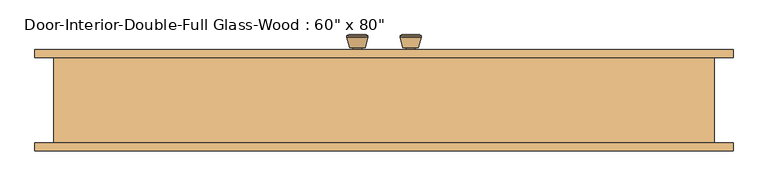
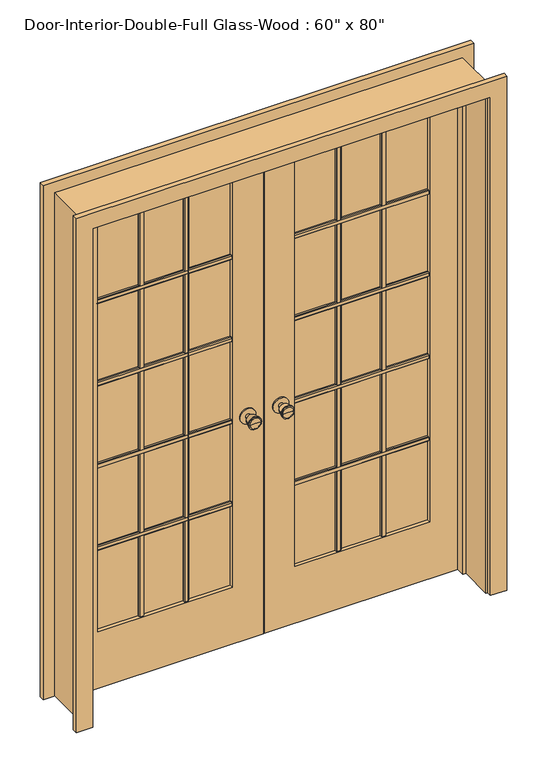
"""IFC4 building model written with IfcOpenShell, lengths in millimetres: door geometry."""

from ifc_helpers import new_model, si_unit, point, frame, frame_2d, origin, place, context, project, spatial, polyline, circle_curve, trimmed, segment, composite_curve, outline, extrude, faceted_brep, source, transform, mapped, element, save
from ifc_brep_helpers import plane_surface, cylinder_surface, revolved_surface, advanced_brep


def door_9d00318c(model_context):
    return source(origin(), model_context, "Body", "SolidModel", [
        advanced_brep(
        [(-63.5, 104.425, 914.4), (-73.5, 104.425, 914.4), (-53.5, 104.425, 914.4), (-83.9758676, 153.425, 914.4), (-63.5, 153.425, 914.4), (-43.0241324, 153.425, 914.4), (-88.5, 151.5971319, 914.4), (-38.5, 151.5971319, 914.4), (-88.5, 148.1334537, 914.4), (-38.5, 148.1334537, 914.4), (-82.136236, 123.425, 914.4), (-44.863764, 123.425, 914.4), (-73.5, 123.425, 914.4), (-53.5, 123.425, 914.4)],
        [
            (0, 1),
            (1, 2, circle_curve(frame((-63.5, 104.425, 914.4), z_axis=(0.0, -1.0, 0.0), x_axis=(1.0, 0.0, 0.0)), 10.0)),
            (2, 0),
            (2, 1, circle_curve(frame((-63.5, 104.425, 914.4), z_axis=(0.0, -1.0, 0.0), x_axis=(1.0, 0.0, 0.0)), 10.0)),
            (3, 4),
            (4, 5),
            (5, 3, circle_curve(frame((-63.5, 153.425, 914.4), z_axis=(0.0, 1.0, 0.0), x_axis=(1.0, 0.0, 0.0)), 20.4758676)),
            (3, 5, circle_curve(frame((-63.5, 153.425, 914.4), z_axis=(0.0, 1.0, 0.0), x_axis=(1.0, 0.0, 0.0)), 20.4758676)),
            (6, 3),
            (5, 7),
            (7, 6, circle_curve(frame((-63.5, 151.5971319, 914.4), z_axis=(0.0, 1.0, 0.0), x_axis=(1.0, 0.0, 0.0)), 25.0)),
            (6, 7, circle_curve(frame((-63.5, 151.5971319, 914.4), z_axis=(0.0, 1.0, 0.0), x_axis=(1.0, 0.0, 0.0)), 25.0)),
            (8, 6),
            (7, 9),
            (9, 8, circle_curve(frame((-63.5, 148.1334537, 914.4), z_axis=(0.0, 1.0, 0.0), x_axis=(1.0, 0.0, 0.0)), 25.0)),
            (8, 9, circle_curve(frame((-63.5, 148.1334537, 914.4), z_axis=(0.0, 1.0, 0.0), x_axis=(1.0, 0.0, 0.0)), 25.0)),
            (10, 8),
            (9, 11),
            (11, 10, circle_curve(frame((-63.5, 123.425, 914.4), z_axis=(0.0, 1.0, 0.0), x_axis=(1.0, 0.0, 0.0)), 18.636236)),
            (10, 11, circle_curve(frame((-63.5, 123.425, 914.4), z_axis=(0.0, 1.0, 0.0), x_axis=(1.0, 0.0, 0.0)), 18.636236)),
            (12, 10),
            (11, 13),
            (13, 12, circle_curve(frame((-63.5, 123.425, 914.4), z_axis=(0.0, 1.0, 0.0), x_axis=(1.0, 0.0, 0.0)), 10.0)),
            (12, 13, circle_curve(frame((-63.5, 123.425, 914.4), z_axis=(0.0, 1.0, 0.0), x_axis=(1.0, 0.0, 0.0)), 10.0)),
            (1, 12),
            (13, 2),
        ],
        [
            plane_surface(frame((-63.5, 104.425, 914.4), z_axis=(0.0, -1.0, 0.0), x_axis=(1.0, 0.0, 0.0))),
            plane_surface(frame((-63.5, 153.425, 914.4), z_axis=(0.0, 1.0, 0.0), x_axis=(1.0, 0.0, 0.0))),
            revolved_surface(polyline([(-43.0241324, 153.425, 914.4), (-38.5, 151.5971319, 914.4)]), (-63.5, 104.425, 914.4), (0.0, -1.0, 0.0)),
            cylinder_surface(frame((-63.5, 104.425, 914.4), z_axis=(0.0, -1.0, 0.0), x_axis=(1.0, 0.0, 0.0)), 25.0),
            revolved_surface(polyline([(-38.5, 148.1334537, 914.4), (-44.863764, 123.425, 914.4)]), (-63.5, 104.425, 914.4), (0.0, -1.0, 0.0)),
            plane_surface(frame((-63.5, 123.425, 914.4), z_axis=(0.0, -1.0, 0.0), x_axis=(1.0, 0.0, 0.0))),
            cylinder_surface(frame((-63.5, 104.425, 914.4), z_axis=(0.0, -1.0, 0.0), x_axis=(1.0, 0.0, 0.0)), 10.0),
        ],
        [
            (0, [[1, 2, 3]]),
            (0, [[-3, 4, -1]]),
            (1, [[5, 6, 7]]),
            (1, [[-6, -5, 8]]),
            (2, [[9, -7, 10, 11]]),
            (2, [[-10, -8, -9, 12]]),
            (3, [[13, -11, 14, 15]]),
            (3, [[-14, -12, -13, 16]]),
            (4, [[17, -15, 18, 19]]),
            (4, [[-18, -16, -17, 20]]),
            (5, [[21, -19, 22, 23]]),
            (5, [[-22, -20, -21, 24]]),
            (6, [[25, -23, 26, -2]]),
            (6, [[-26, -24, -25, -4]]),
        ],
    ),
        extrude(outline(composite_curve([segment(trimmed(circle_curve(frame_2d((914.4, -63.5)), 30.0), [point((914.4, -33.5))], [point((914.4, -93.5))], False, "CARTESIAN"), True, "CONTINUOUS"), segment(trimmed(circle_curve(frame_2d((914.4, -63.5)), 30.0), [point((914.4, -93.5))], [point((914.4, -33.5))], False, "CARTESIAN"), True, "CONTINUOUS")], self_intersect=False)), frame((0.0, 98.425, 0.0), z_axis=(0.0, 1.0, 0.0), x_axis=(0.0, 0.0, 1.0)), (0.0, 0.0, 1.0), 6.0),
        advanced_brep(
        [(-63.5, 57.5, 914.4), (-53.5, 57.5, 914.4), (-73.5, 57.5, 914.4), (-83.9758676, 8.5, 914.4), (-43.0241324, 8.5, 914.4), (-63.5, 8.5, 914.4), (-88.5, 10.3278681, 914.4), (-38.5, 10.3278681, 914.4), (-88.5, 13.7915463, 914.4), (-38.5, 13.7915463, 914.4), (-82.136236, 38.5, 914.4), (-44.863764, 38.5, 914.4), (-73.5, 38.5, 914.4), (-53.5, 38.5, 914.4)],
        [
            (0, 1),
            (1, 2, circle_curve(frame((-63.5, 57.5, 914.4), z_axis=(0.0, 1.0, 0.0), x_axis=(1.0, 0.0, 0.0)), 10.0)),
            (2, 0),
            (2, 1, circle_curve(frame((-63.5, 57.5, 914.4), z_axis=(0.0, 1.0, 0.0), x_axis=(1.0, 0.0, 0.0)), 10.0)),
            (3, 4, circle_curve(frame((-63.5, 8.5, 914.4), z_axis=(0.0, -1.0, 0.0), x_axis=(1.0, 0.0, 0.0)), 20.4758676)),
            (4, 5),
            (5, 3),
            (4, 3, circle_curve(frame((-63.5, 8.5, 914.4), z_axis=(0.0, -1.0, 0.0), x_axis=(1.0, 0.0, 0.0)), 20.4758676)),
            (6, 7, circle_curve(frame((-63.5, 10.3278681, 914.4), z_axis=(0.0, -1.0, 0.0), x_axis=(1.0, 0.0, 0.0)), 25.0)),
            (7, 4),
            (3, 6),
            (7, 6, circle_curve(frame((-63.5, 10.3278681, 914.4), z_axis=(0.0, -1.0, 0.0), x_axis=(1.0, 0.0, 0.0)), 25.0)),
            (8, 9, circle_curve(frame((-63.5, 13.7915463, 914.4), z_axis=(0.0, -1.0, 0.0), x_axis=(1.0, 0.0, 0.0)), 25.0)),
            (9, 7),
            (6, 8),
            (9, 8, circle_curve(frame((-63.5, 13.7915463, 914.4), z_axis=(0.0, -1.0, 0.0), x_axis=(1.0, 0.0, 0.0)), 25.0)),
            (10, 11, circle_curve(frame((-63.5, 38.5, 914.4), z_axis=(0.0, -1.0, 0.0), x_axis=(1.0, 0.0, 0.0)), 18.636236)),
            (11, 9),
            (8, 10),
            (11, 10, circle_curve(frame((-63.5, 38.5, 914.4), z_axis=(0.0, -1.0, 0.0), x_axis=(1.0, 0.0, 0.0)), 18.636236)),
            (12, 13, circle_curve(frame((-63.5, 38.5, 914.4), z_axis=(0.0, -1.0, 0.0), x_axis=(1.0, 0.0, 0.0)), 10.0)),
            (13, 11),
            (10, 12),
            (13, 12, circle_curve(frame((-63.5, 38.5, 914.4), z_axis=(0.0, -1.0, 0.0), x_axis=(1.0, 0.0, 0.0)), 10.0)),
            (1, 13),
            (12, 2),
        ],
        [
            plane_surface(frame((-63.5, 57.5, 914.4), z_axis=(0.0, 1.0, 0.0), x_axis=(1.0, 0.0, 0.0))),
            plane_surface(frame((-63.5, 8.5, 914.4), z_axis=(0.0, -1.0, 0.0), x_axis=(1.0, 0.0, 0.0))),
            revolved_surface(polyline([(-43.0241324, 8.5, 914.4), (-38.5, 10.3278681, 914.4)]), (-63.5, 57.5, 914.4), (0.0, 1.0, 0.0)),
            cylinder_surface(frame((-63.5, 57.5, 914.4), z_axis=(0.0, 1.0, 0.0), x_axis=(1.0, 0.0, 0.0)), 25.0),
            revolved_surface(polyline([(-38.5, 13.7915463, 914.4), (-44.863764, 38.5, 914.4)]), (-63.5, 57.5, 914.4), (0.0, 1.0, 0.0)),
            plane_surface(frame((-63.5, 38.5, 914.4), z_axis=(0.0, 1.0, 0.0), x_axis=(1.0, 0.0, 0.0))),
            cylinder_surface(frame((-63.5, 57.5, 914.4), z_axis=(0.0, 1.0, 0.0), x_axis=(1.0, 0.0, 0.0)), 10.0),
        ],
        [
            (0, [[1, 2, 3]]),
            (0, [[-3, 4, -1]]),
            (1, [[5, 6, 7]]),
            (1, [[8, -7, -6]]),
            (2, [[9, 10, -5, 11]]),
            (2, [[12, -11, -8, -10]]),
            (3, [[13, 14, -9, 15]]),
            (3, [[16, -15, -12, -14]]),
            (4, [[17, 18, -13, 19]]),
            (4, [[20, -19, -16, -18]]),
            (5, [[21, 22, -17, 23]]),
            (5, [[24, -23, -20, -22]]),
            (6, [[-2, 25, -21, 26]]),
            (6, [[-4, -26, -24, -25]]),
        ],
    ),
        extrude(outline(composite_curve([segment(trimmed(circle_curve(frame_2d((914.4, -63.5)), 30.0), [point((914.4, -33.5))], [point((914.4, -93.5))], False, "CARTESIAN"), True, "CONTINUOUS"), segment(trimmed(circle_curve(frame_2d((914.4, -63.5)), 30.0), [point((914.4, -93.5))], [point((914.4, -33.5))], False, "CARTESIAN"), True, "CONTINUOUS")], self_intersect=False)), frame((0.0, 57.5, 0.0), z_axis=(0.0, 1.0, 0.0), x_axis=(0.0, 0.0, 1.0)), (0.0, 0.0, 1.0), 6.0),
        extrude(outline(polyline([(77.47, 1586.23), (77.47, 1567.18), (71.12, 1567.18), (67.945, 1570.355), (67.945, 1583.055), (71.12, 1586.23), (77.47, 1586.23)])), frame((120.65, 0.0, 0.0), z_axis=(1.0, 0.0, 0.0), x_axis=(0.0, 1.0, 0.0)), (0.0, 0.0, 1.0), 520.7),
        extrude(outline(polyline([(77.47, 1249.9975), (77.47, 1230.9475), (71.12, 1230.9475), (67.945, 1234.1225), (67.945, 1246.8225), (71.12, 1249.9975), (77.47, 1249.9975)])), frame((120.65, 0.0, 0.0), z_axis=(1.0, 0.0, 0.0), x_axis=(0.0, 1.0, 0.0)), (0.0, 0.0, 1.0), 520.7),
        extrude(outline(polyline([(77.47, 913.765), (77.47, 894.715), (71.12, 894.715), (67.945, 897.89), (67.945, 910.59), (71.12, 913.765), (77.47, 913.765)])), frame((120.65, 0.0, 0.0), z_axis=(1.0, 0.0, 0.0), x_axis=(0.0, 1.0, 0.0)), (0.0, 0.0, 1.0), 520.7),
        extrude(outline(polyline([(77.47, 577.5325), (77.47, 558.4825), (71.12, 558.4825), (67.945, 561.6575), (67.945, 574.3575), (71.12, 577.5325), (77.47, 577.5325)])), frame((120.65, 0.0, 0.0), z_axis=(1.0, 0.0, 0.0), x_axis=(0.0, 1.0, 0.0)), (0.0, 0.0, 1.0), 520.7),
        extrude(outline(polyline([(458.2583333, 77.47), (477.3083333, 77.47), (477.3083333, 71.12), (474.1333333, 67.945), (461.4333333, 67.945), (458.2583333, 71.12), (458.2583333, 77.47)])), frame((0.0, 0.0, 231.775), z_axis=(0.0, 0.0, 1.0), x_axis=(1.0, 0.0, 0.0)), (0.0, 0.0, 1.0), 1681.1625),
        extrude(outline(polyline([(284.6916667, 77.47), (303.7416667, 77.47), (303.7416667, 71.12), (300.5666667, 67.945), (287.8666667, 67.945), (284.6916667, 71.12), (284.6916667, 77.47)])), frame((0.0, 0.0, 231.775), z_axis=(0.0, 0.0, 1.0), x_axis=(1.0, 0.0, 0.0)), (0.0, 0.0, 1.0), 1681.1625),
        extrude(outline(polyline([(84.455, 1586.23), (90.805, 1586.23), (93.98, 1583.055), (93.98, 1570.355), (90.805, 1567.18), (84.455, 1567.18), (84.455, 1586.23)])), frame((-641.35, 0.0, 0.0), z_axis=(1.0, 0.0, 0.0), x_axis=(0.0, 1.0, 0.0)), (0.0, 0.0, 1.0), 520.7),
        extrude(outline(polyline([(84.455, 1249.9975), (90.805, 1249.9975), (93.98, 1246.8225), (93.98, 1234.1225), (90.805, 1230.9475), (84.455, 1230.9475), (84.455, 1249.9975)])), frame((-641.35, 0.0, 0.0), z_axis=(1.0, 0.0, 0.0), x_axis=(0.0, 1.0, 0.0)), (0.0, 0.0, 1.0), 520.7),
        extrude(outline(polyline([(84.455, 913.765), (90.805, 913.765), (93.98, 910.59), (93.98, 897.89), (90.805, 894.715), (84.455, 894.715), (84.455, 913.765)])), frame((-641.35, 0.0, 0.0), z_axis=(1.0, 0.0, 0.0), x_axis=(0.0, 1.0, 0.0)), (0.0, 0.0, 1.0), 520.7),
        extrude(outline(polyline([(84.455, 577.5325), (90.805, 577.5325), (93.98, 574.3575), (93.98, 561.6575), (90.805, 558.4825), (84.455, 558.4825), (84.455, 577.5325)])), frame((-641.35, 0.0, 0.0), z_axis=(1.0, 0.0, 0.0), x_axis=(0.0, 1.0, 0.0)), (0.0, 0.0, 1.0), 520.7),
        extrude(outline(polyline([(-303.7416667, 84.455), (-303.7416667, 90.805), (-300.5666667, 93.98), (-287.8666667, 93.98), (-284.6916667, 90.805), (-284.6916667, 84.455), (-303.7416667, 84.455)])), frame((0.0, 0.0, 231.775), z_axis=(0.0, 0.0, 1.0), x_axis=(1.0, 0.0, 0.0)), (0.0, 0.0, 1.0), 1681.1625),
        extrude(outline(polyline([(-477.3083333, 84.455), (-477.3083333, 90.805), (-474.1333333, 93.98), (-461.4333333, 93.98), (-458.2583333, 90.805), (-458.2583333, 84.455), (-477.3083333, 84.455)])), frame((0.0, 0.0, 231.775), z_axis=(0.0, 0.0, 1.0), x_axis=(1.0, 0.0, 0.0)), (0.0, 0.0, 1.0), 1681.1625),
        extrude(outline(polyline([(84.455, 1586.23), (90.805, 1586.23), (93.98, 1583.055), (93.98, 1570.355), (90.805, 1567.18), (84.455, 1567.18), (84.455, 1586.23)])), frame((120.65, 0.0, 0.0), z_axis=(1.0, 0.0, 0.0), x_axis=(0.0, 1.0, 0.0)), (0.0, 0.0, 1.0), 520.7),
        extrude(outline(polyline([(84.455, 1249.9975), (90.805, 1249.9975), (93.98, 1246.8225), (93.98, 1234.1225), (90.805, 1230.9475), (84.455, 1230.9475), (84.455, 1249.9975)])), frame((120.65, 0.0, 0.0), z_axis=(1.0, 0.0, 0.0), x_axis=(0.0, 1.0, 0.0)), (0.0, 0.0, 1.0), 520.7),
        extrude(outline(polyline([(84.455, 913.765), (90.805, 913.765), (93.98, 910.59), (93.98, 897.89), (90.805, 894.715), (84.455, 894.715), (84.455, 913.765)])), frame((120.65, 0.0, 0.0), z_axis=(1.0, 0.0, 0.0), x_axis=(0.0, 1.0, 0.0)), (0.0, 0.0, 1.0), 520.7),
        extrude(outline(polyline([(84.455, 577.5325), (90.805, 577.5325), (93.98, 574.3575), (93.98, 561.6575), (90.805, 558.4825), (84.455, 558.4825), (84.455, 577.5325)])), frame((120.65, 0.0, 0.0), z_axis=(1.0, 0.0, 0.0), x_axis=(0.0, 1.0, 0.0)), (0.0, 0.0, 1.0), 520.7),
        extrude(outline(polyline([(458.2583333, 84.455), (458.2583333, 90.805), (461.4333333, 93.98), (474.1333333, 93.98), (477.3083333, 90.805), (477.3083333, 84.455), (458.2583333, 84.455)])), frame((0.0, 0.0, 231.775), z_axis=(0.0, 0.0, 1.0), x_axis=(1.0, 0.0, 0.0)), (0.0, 0.0, 1.0), 1681.1625),
        extrude(outline(polyline([(284.6916667, 84.455), (284.6916667, 90.805), (287.8666667, 93.98), (300.5666667, 93.98), (303.7416667, 90.805), (303.7416667, 84.455), (284.6916667, 84.455)])), frame((0.0, 0.0, 231.775), z_axis=(0.0, 0.0, 1.0), x_axis=(1.0, 0.0, 0.0)), (0.0, 0.0, 1.0), 1681.1625),
        extrude(outline(polyline([(77.47, 1586.23), (77.47, 1567.18), (71.12, 1567.18), (67.945, 1570.355), (67.945, 1583.055), (71.12, 1586.23), (77.47, 1586.23)])), frame((-641.35, 0.0, 0.0), z_axis=(1.0, 0.0, 0.0), x_axis=(0.0, 1.0, 0.0)), (0.0, 0.0, 1.0), 520.7),
        extrude(outline(polyline([(77.47, 1249.9975), (77.47, 1230.9475), (71.12, 1230.9475), (67.945, 1234.1225), (67.945, 1246.8225), (71.12, 1249.9975), (77.47, 1249.9975)])), frame((-641.35, 0.0, 0.0), z_axis=(1.0, 0.0, 0.0), x_axis=(0.0, 1.0, 0.0)), (0.0, 0.0, 1.0), 520.7),
        extrude(outline(polyline([(77.47, 913.765), (77.47, 894.715), (71.12, 894.715), (67.945, 897.89), (67.945, 910.59), (71.12, 913.765), (77.47, 913.765)])), frame((-641.35, 0.0, 0.0), z_axis=(1.0, 0.0, 0.0), x_axis=(0.0, 1.0, 0.0)), (0.0, 0.0, 1.0), 520.7),
        extrude(outline(polyline([(77.47, 577.5325), (77.47, 558.4825), (71.12, 558.4825), (67.945, 561.6575), (67.945, 574.3575), (71.12, 577.5325), (77.47, 577.5325)])), frame((-641.35, 0.0, 0.0), z_axis=(1.0, 0.0, 0.0), x_axis=(0.0, 1.0, 0.0)), (0.0, 0.0, 1.0), 520.7),
        extrude(outline(polyline([(-303.7416667, 77.47), (-284.6916667, 77.47), (-284.6916667, 71.12), (-287.8666667, 67.945), (-300.5666667, 67.945), (-303.7416667, 71.12), (-303.7416667, 77.47)])), frame((0.0, 0.0, 231.775), z_axis=(0.0, 0.0, 1.0), x_axis=(1.0, 0.0, 0.0)), (0.0, 0.0, 1.0), 1681.1625),
        extrude(outline(polyline([(-477.3083333, 77.47), (-458.2583333, 77.47), (-458.2583333, 71.12), (-461.4333333, 67.945), (-474.1333333, 67.945), (-477.3083333, 71.12), (-477.3083333, 77.47)])), frame((0.0, 0.0, 231.775), z_axis=(0.0, 0.0, 1.0), x_axis=(1.0, 0.0, 0.0)), (0.0, 0.0, 1.0), 1681.1625),
        advanced_brep(
        [(63.5, 57.5, 914.4), (73.5, 57.5, 914.4), (53.5, 57.5, 914.4), (83.9758676, 8.5, 914.4), (63.5, 8.5, 914.4), (43.0241324, 8.5, 914.4), (88.5, 10.3278681, 914.4), (38.5, 10.3278681, 914.4), (88.5, 13.7915463, 914.4), (38.5, 13.7915463, 914.4), (82.136236, 38.5, 914.4), (44.863764, 38.5, 914.4), (73.5, 38.5, 914.4), (53.5, 38.5, 914.4)],
        [
            (0, 1),
            (1, 2, circle_curve(frame((63.5, 57.5, 914.4), z_axis=(0.0, 1.0, 0.0), x_axis=(-1.0, 0.0, 0.0)), 10.0)),
            (2, 0),
            (2, 1, circle_curve(frame((63.5, 57.5, 914.4), z_axis=(0.0, 1.0, 0.0), x_axis=(-1.0, 0.0, 0.0)), 10.0)),
            (3, 4),
            (4, 5),
            (5, 3, circle_curve(frame((63.5, 8.5, 914.4), z_axis=(0.0, -1.0, 0.0), x_axis=(-1.0, 0.0, 0.0)), 20.4758676)),
            (3, 5, circle_curve(frame((63.5, 8.5, 914.4), z_axis=(0.0, -1.0, 0.0), x_axis=(-1.0, 0.0, 0.0)), 20.4758676)),
            (6, 3),
            (5, 7),
            (7, 6, circle_curve(frame((63.5, 10.3278681, 914.4), z_axis=(0.0, -1.0, 0.0), x_axis=(-1.0, 0.0, 0.0)), 25.0)),
            (6, 7, circle_curve(frame((63.5, 10.3278681, 914.4), z_axis=(0.0, -1.0, 0.0), x_axis=(-1.0, 0.0, 0.0)), 25.0)),
            (8, 6),
            (7, 9),
            (9, 8, circle_curve(frame((63.5, 13.7915463, 914.4), z_axis=(0.0, -1.0, 0.0), x_axis=(-1.0, 0.0, 0.0)), 25.0)),
            (8, 9, circle_curve(frame((63.5, 13.7915463, 914.4), z_axis=(0.0, -1.0, 0.0), x_axis=(-1.0, 0.0, 0.0)), 25.0)),
            (10, 8),
            (9, 11),
            (11, 10, circle_curve(frame((63.5, 38.5, 914.4), z_axis=(0.0, -1.0, 0.0), x_axis=(-1.0, 0.0, 0.0)), 18.636236)),
            (10, 11, circle_curve(frame((63.5, 38.5, 914.4), z_axis=(0.0, -1.0, 0.0), x_axis=(-1.0, 0.0, 0.0)), 18.636236)),
            (12, 10),
            (11, 13),
            (13, 12, circle_curve(frame((63.5, 38.5, 914.4), z_axis=(0.0, -1.0, 0.0), x_axis=(-1.0, 0.0, 0.0)), 10.0)),
            (12, 13, circle_curve(frame((63.5, 38.5, 914.4), z_axis=(0.0, -1.0, 0.0), x_axis=(-1.0, 0.0, 0.0)), 10.0)),
            (1, 12),
            (13, 2),
        ],
        [
            plane_surface(frame((63.5, 57.5, 914.4), z_axis=(0.0, 1.0, 0.0), x_axis=(-1.0, 0.0, 0.0))),
            plane_surface(frame((63.5, 8.5, 914.4), z_axis=(0.0, -1.0, 0.0), x_axis=(-1.0, 0.0, 0.0))),
            revolved_surface(polyline([(43.0241324, 8.5, 914.4), (38.5, 10.3278681, 914.4)]), (63.5, 57.5, 914.4), (0.0, 1.0, 0.0)),
            cylinder_surface(frame((63.5, 57.5, 914.4), z_axis=(0.0, 1.0, 0.0), x_axis=(-1.0, 0.0, 0.0)), 25.0),
            revolved_surface(polyline([(38.5, 13.7915463, 914.4), (44.863764, 38.5, 914.4)]), (63.5, 57.5, 914.4), (0.0, 1.0, 0.0)),
            plane_surface(frame((63.5, 38.5, 914.4), z_axis=(0.0, 1.0, 0.0), x_axis=(-1.0, 0.0, 0.0))),
            cylinder_surface(frame((63.5, 57.5, 914.4), z_axis=(0.0, 1.0, 0.0), x_axis=(-1.0, 0.0, 0.0)), 10.0),
        ],
        [
            (0, [[1, 2, 3]]),
            (0, [[-3, 4, -1]]),
            (1, [[5, 6, 7]]),
            (1, [[-6, -5, 8]]),
            (2, [[9, -7, 10, 11]]),
            (2, [[-10, -8, -9, 12]]),
            (3, [[13, -11, 14, 15]]),
            (3, [[-14, -12, -13, 16]]),
            (4, [[17, -15, 18, 19]]),
            (4, [[-18, -16, -17, 20]]),
            (5, [[21, -19, 22, 23]]),
            (5, [[-22, -20, -21, 24]]),
            (6, [[25, -23, 26, -2]]),
            (6, [[-26, -24, -25, -4]]),
        ],
    ),
        extrude(outline(composite_curve([segment(trimmed(circle_curve(frame_2d((914.4, 63.5)), 30.0), [point((914.4, 33.5))], [point((914.4, 93.5))], False, "CARTESIAN"), True, "CONTINUOUS"), segment(trimmed(circle_curve(frame_2d((914.4, 63.5)), 30.0), [point((914.4, 93.5))], [point((914.4, 33.5))], False, "CARTESIAN"), True, "CONTINUOUS")], self_intersect=False)), frame((0.0, 57.5, 0.0), z_axis=(0.0, 1.0, 0.0), x_axis=(0.0, 0.0, 1.0)), (0.0, 0.0, 1.0), 6.0),
        advanced_brep(
        [(63.5, 104.425, 914.4), (53.5, 104.425, 914.4), (73.5, 104.425, 914.4), (83.9758676, 153.425, 914.4), (43.0241324, 153.425, 914.4), (63.5, 153.425, 914.4), (88.5, 151.5971319, 914.4), (38.5, 151.5971319, 914.4), (88.5, 148.1334537, 914.4), (38.5, 148.1334537, 914.4), (82.136236, 123.425, 914.4), (44.863764, 123.425, 914.4), (73.5, 123.425, 914.4), (53.5, 123.425, 914.4)],
        [
            (0, 1),
            (1, 2, circle_curve(frame((63.5, 104.425, 914.4), z_axis=(0.0, -1.0, 0.0), x_axis=(-1.0, 0.0, 0.0)), 10.0)),
            (2, 0),
            (2, 1, circle_curve(frame((63.5, 104.425, 914.4), z_axis=(0.0, -1.0, 0.0), x_axis=(-1.0, 0.0, 0.0)), 10.0)),
            (3, 4, circle_curve(frame((63.5, 153.425, 914.4), z_axis=(0.0, 1.0, 0.0), x_axis=(-1.0, 0.0, 0.0)), 20.4758676)),
            (4, 5),
            (5, 3),
            (4, 3, circle_curve(frame((63.5, 153.425, 914.4), z_axis=(0.0, 1.0, 0.0), x_axis=(-1.0, 0.0, 0.0)), 20.4758676)),
            (6, 7, circle_curve(frame((63.5, 151.5971319, 914.4), z_axis=(0.0, 1.0, 0.0), x_axis=(-1.0, 0.0, 0.0)), 25.0)),
            (7, 4),
            (3, 6),
            (7, 6, circle_curve(frame((63.5, 151.5971319, 914.4), z_axis=(0.0, 1.0, 0.0), x_axis=(-1.0, 0.0, 0.0)), 25.0)),
            (8, 9, circle_curve(frame((63.5, 148.1334537, 914.4), z_axis=(0.0, 1.0, 0.0), x_axis=(-1.0, 0.0, 0.0)), 25.0)),
            (9, 7),
            (6, 8),
            (9, 8, circle_curve(frame((63.5, 148.1334537, 914.4), z_axis=(0.0, 1.0, 0.0), x_axis=(-1.0, 0.0, 0.0)), 25.0)),
            (10, 11, circle_curve(frame((63.5, 123.425, 914.4), z_axis=(0.0, 1.0, 0.0), x_axis=(-1.0, 0.0, 0.0)), 18.636236)),
            (11, 9),
            (8, 10),
            (11, 10, circle_curve(frame((63.5, 123.425, 914.4), z_axis=(0.0, 1.0, 0.0), x_axis=(-1.0, 0.0, 0.0)), 18.636236)),
            (12, 13, circle_curve(frame((63.5, 123.425, 914.4), z_axis=(0.0, 1.0, 0.0), x_axis=(-1.0, 0.0, 0.0)), 10.0)),
            (13, 11),
            (10, 12),
            (13, 12, circle_curve(frame((63.5, 123.425, 914.4), z_axis=(0.0, 1.0, 0.0), x_axis=(-1.0, 0.0, 0.0)), 10.0)),
            (1, 13),
            (12, 2),
        ],
        [
            plane_surface(frame((63.5, 104.425, 914.4), z_axis=(0.0, -1.0, 0.0), x_axis=(-1.0, 0.0, 0.0))),
            plane_surface(frame((63.5, 153.425, 914.4), z_axis=(0.0, 1.0, 0.0), x_axis=(-1.0, 0.0, 0.0))),
            revolved_surface(polyline([(43.0241324, 153.425, 914.4), (38.5, 151.5971319, 914.4)]), (63.5, 104.425, 914.4), (0.0, -1.0, 0.0)),
            cylinder_surface(frame((63.5, 104.425, 914.4), z_axis=(0.0, -1.0, 0.0), x_axis=(-1.0, 0.0, 0.0)), 25.0),
            revolved_surface(polyline([(38.5, 148.1334537, 914.4), (44.863764, 123.425, 914.4)]), (63.5, 104.425, 914.4), (0.0, -1.0, 0.0)),
            plane_surface(frame((63.5, 123.425, 914.4), z_axis=(0.0, -1.0, 0.0), x_axis=(-1.0, 0.0, 0.0))),
            cylinder_surface(frame((63.5, 104.425, 914.4), z_axis=(0.0, -1.0, 0.0), x_axis=(-1.0, 0.0, 0.0)), 10.0),
        ],
        [
            (0, [[1, 2, 3]]),
            (0, [[-3, 4, -1]]),
            (1, [[5, 6, 7]]),
            (1, [[8, -7, -6]]),
            (2, [[9, 10, -5, 11]]),
            (2, [[12, -11, -8, -10]]),
            (3, [[13, 14, -9, 15]]),
            (3, [[16, -15, -12, -14]]),
            (4, [[17, 18, -13, 19]]),
            (4, [[20, -19, -16, -18]]),
            (5, [[21, 22, -17, 23]]),
            (5, [[24, -23, -20, -22]]),
            (6, [[-2, 25, -21, 26]]),
            (6, [[-4, -26, -24, -25]]),
        ],
    ),
        extrude(outline(composite_curve([segment(trimmed(circle_curve(frame_2d((914.4, 63.5)), 30.0), [point((914.4, 33.5))], [point((914.4, 93.5))], False, "CARTESIAN"), True, "CONTINUOUS"), segment(trimmed(circle_curve(frame_2d((914.4, 63.5)), 30.0), [point((914.4, 93.5))], [point((914.4, 33.5))], False, "CARTESIAN"), True, "CONTINUOUS")], self_intersect=False)), frame((0.0, 98.425, 0.0), z_axis=(0.0, 1.0, 0.0), x_axis=(0.0, 0.0, 1.0)), (0.0, 0.0, 1.0), 6.0),
        extrude(outline(polyline([(0.0, 768.35), (0.0, 831.85), (2101.85, 831.85), (2101.85, -831.85), (0.0, -831.85), (0.0, -768.35), (2038.35, -768.35), (2038.35, 768.35), (0.0, 768.35)])), frame((0.0, 98.425, 0.0), z_axis=(0.0, 1.0, 0.0), x_axis=(0.0, 0.0, 1.0)), (0.0, 0.0, 1.0), 19.05),
        extrude(outline(polyline([(0.0, 768.35), (0.0, 831.85), (2101.85, 831.85), (2101.85, -831.85), (0.0, -831.85), (0.0, -768.35), (2038.35, -768.35), (2038.35, 768.35), (0.0, 768.35)])), frame((0.0, -123.825, 0.0), z_axis=(0.0, 1.0, 0.0), x_axis=(0.0, 0.0, 1.0)), (0.0, 0.0, 1.0), 19.05),
        extrude(outline(polyline([(2032.0, -762.0), (0.0, -762.0), (0.0, -1.6019111), (2032.0, -1.6019111), (2032.0, -762.0)]), holes=[polyline([(231.775, -641.35), (1912.9375, -641.35), (1912.9375, -120.65), (231.775, -120.65), (231.775, -641.35)])]), frame((0.0, 63.5, 0.0), z_axis=(0.0, 1.0, 0.0), x_axis=(0.0, 0.0, 1.0)), (0.0, 0.0, 1.0), 34.925),
        extrude(outline(polyline([(0.0, 762.0), (2032.0, 762.0), (2032.0, 1.5875), (0.0, 1.5875), (0.0, 762.0)]), holes=[polyline([(1912.9375, 120.65), (1912.9375, 641.35), (231.775, 641.35), (231.775, 120.65), (1912.9375, 120.65)])]), frame((0.0, 63.5, 0.0), z_axis=(0.0, 1.0, 0.0), x_axis=(0.0, 0.0, 1.0)), (0.0, 0.0, 1.0), 34.925),
        faceted_brep([(787.4, 98.425, 0.0), (787.4, -104.775, 0.0), (762.0, -104.775, 0.0), (762.0, 28.575, 0.0), (749.3, 28.575, 0.0), (749.3, 63.5, 0.0), (762.0, 63.5, 0.0), (762.0, 98.425, 0.0), (787.4, 98.425, 2057.4), (787.4, -104.775, 2057.4), (-787.4, -104.775, 2057.4), (-787.4, -104.775, 0.0), (-762.0, -104.775, 0.0), (-762.0, -104.775, 2032.0), (762.0, -104.775, 2032.0), (762.0, 28.575, 2032.0), (-762.0, 28.575, 2032.0), (-762.0, 28.575, 0.0), (-749.3, 28.575, 0.0), (-749.3, 28.575, 2019.3), (749.3, 28.575, 2019.3), (749.3, 63.5, 2019.3), (1.5875, 63.5, 2019.3), (-1.6019111, 63.5, 2019.3), (-749.3, 63.5, 2019.3), (-749.3, 63.5, 0.0), (-762.0, 63.5, 0.0), (-762.0, 63.5, 2032.0), (-1.6019111, 63.5, 2032.0), (1.5875, 63.5, 2032.0), (762.0, 63.5, 2032.0), (762.0, 98.425, 2032.0), (1.5875, 98.425, 2032.0), (-1.6019111, 98.425, 2032.0), (-762.0, 98.425, 2032.0), (-762.0, 98.425, 0.0), (-787.4, 98.425, 0.0), (-787.4, 98.425, 2057.4)], [[[0, 1, 2, 3, 4, 5, 6, 7]], [[1, 0, 8, 9]], [[2, 1, 9, 10, 11, 12, 13, 14]], [[3, 2, 14, 15]], [[4, 3, 15, 16, 17, 18, 19, 20]], [[5, 4, 20, 21]], [[6, 5, 21, 22, 23, 24, 25, 26, 27, 28, 29, 30]], [[7, 6, 30, 31]], [[0, 7, 31, 32, 33, 34, 35, 36, 37, 8]], [[9, 8, 37, 10]], [[14, 13, 16, 15]], [[20, 19, 24, 23, 22, 21]], [[31, 30, 29, 28, 27, 34, 33, 32]], [[12, 11, 36, 35, 26, 25, 18, 17]], [[11, 10, 37, 36]], [[13, 12, 17, 16]], [[19, 18, 25, 24]], [[27, 26, 35, 34]]]),
        extrude(outline(polyline([(641.35, 77.47), (120.65, 77.47), (120.65, 84.455), (641.35, 84.455), (641.35, 77.47)])), frame((0.0, 0.0, 231.775), z_axis=(0.0, 0.0, 1.0), x_axis=(1.0, 0.0, 0.0)), (0.0, 0.0, 1.0), 1681.1625),
        extrude(outline(polyline([(-120.65, 77.47), (-641.35, 77.47), (-641.35, 84.455), (-120.65, 84.455), (-120.65, 77.47)])), frame((0.0, 0.0, 231.775), z_axis=(0.0, 0.0, 1.0), x_axis=(1.0, 0.0, 0.0)), (0.0, 0.0, 1.0), 1681.1625),
    ])


if __name__ == "__main__":
    model = new_model("IFC4")
    model_context = context("Model", 3, world=origin())
    ifc_project = project(units=[si_unit("LENGTHUNIT", "METRE", prefix="MILLI")], contexts=[model_context])
    site = spatial("IfcSite", under=ifc_project)
    building = spatial("IfcBuilding", under=site)
    placement = place(None, origin())
    door_shape = door_9d00318c(model_context)
    element("IfcDoor", 1, ObjectType="Door-Interior-Double-Full Glass-Wood : 60\" x 80\"", at=placement, inside=building, context=model_context, shape_type="MappedRepresentation", body=[
        mapped(door_shape, transform((0.0, 0.0, 0.0), x_axis=(1.0, 0.0, 0.0), y_axis=(0.0, 1.0, 0.0), z_axis=(0.0, 0.0, 1.0))),
    ])
    save(model, "model.ifc")

# Revit data of these elements
# Type "Door-Interior-Double-Full Glass-Wood : 60\" x 80\""
#   Type Mark = "10"
#   Assembly Code = "C1020300"
#   Analytic Construction = "French door, wood frame with single glass"
#   Top Rail = 0' - 4 11/16"
#   Thickness = 0' - 1 3/8"
#   Thermal Resistance (R) = 1.0696 (h·ft²·°F)/BTU
#   Swing Angle [instance default] = 90.00°
#   Stiles = 0' - 4 3/4"
#   Rough Width = 5' - 2"
#   Rough Height = 6' - 9"
#   Panel Width = 2' - 6"
#   Height = 6' - 8"
#   Width = 5' - 0"
#   Heat Transfer Coefficient (U) = 0.9350 BTU/(h·ft²·°F)
#   Bottom Rail = 0' - 9 1/8"
#   Show Grill [instance default] = yes
#   Trim Material = Cherry
#   Panel Material = Cherry
#   Frame Material = Cherry
#   Door Handle Material = Aluminum
#   Visual Light Transmittance = 0
#   Solar Heat Gain Coefficient = 0
#   Wall Closure = (empty or 0)
#   Function = (empty or 0)
# Element 1 (IfcDoor, "Door-Interior-Double-Full Glass-Wood : 60\" x 80\"")
#   Materials on its faces: "Cherry", "Aluminum", "Glass"
# Materials
#   "Cherry": class "Wood", colour RGB 226 177 128, transparency 0, Description = "Prunus Serotina", Cost = 0
#   "Aluminum": class "Metal", colour RGB 247 247 247, transparency 0, Description = "Aluminum 6061", Cost = 0
#   "Glass": class "Glass", colour RGB 0 128 192, transparency 0.75, Description = "Soda Lime Glass", Cost = 0
